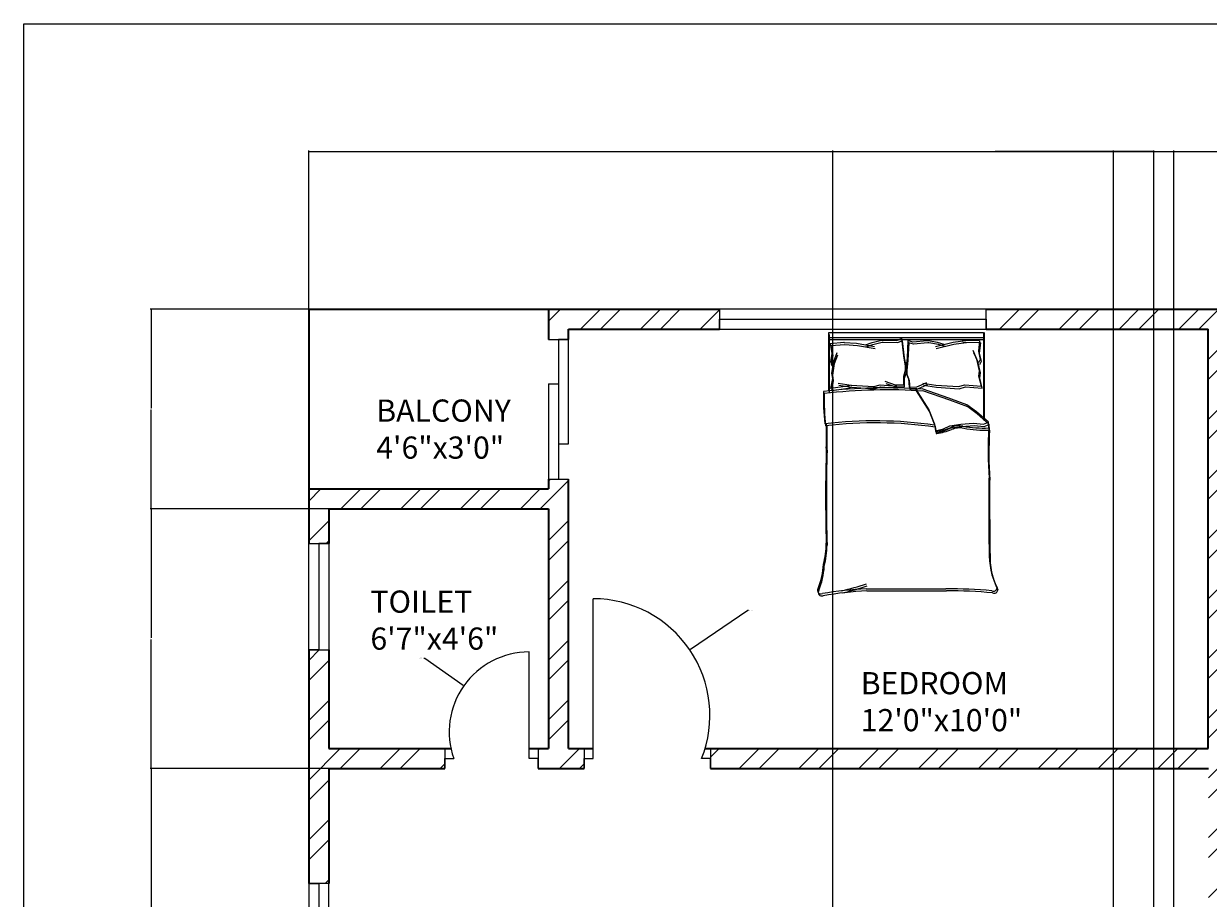
# Model space of a CAD drawing. Units: inches. Extents: x 2064 to 2782, y 1196 to 2299.
# Tile 6 of 11: x 2064 to 2331, y 2102 to 2299. Entities that reach past the tile are written whole.
import ezdxf

# ---------------------------------------------------------------- set-up
doc = ezdxf.new("R2010")
doc.units = ezdxf.units.IN
for name, color, linetype, lineweight in [('A-ANNO-DIMS', 2, 'Continuous', 18), ('A-ANNO-TTLB', 7, 'Continuous', 25), ('A-AREA-IDEN', 7, 'Continuous', 18), ('A-DOOR', 11, 'Continuous', 18), ('A-FURN', 8, 'Continuous', 13), ('A-GLAZ', 151, 'Continuous', 18), ('A-WALL', 7, 'Continuous', 35), ('A-WALL-PATT', 9, 'Continuous', 13)]:
    doc.layers.add(name, color=color, linetype=linetype, lineweight=lineweight)
doc.styles.get("Standard").update_dxf_attribs({"font": 'arial.ttf'})
doc.dimstyles.get("Standard").update_dxf_attribs({"dimtxt": 0.18, "dimasz": 0.18, "dimexe": 0.18, "dimexo": 0.0625, "dimgap": 0.09, "dimtad": 0, "dimtih": 1, "dimtoh": 1, "dimdec": 4, "dimzin": 0, "dimdsep": 46, "dimtxsty": 'Standard', "dimcen": 0.09, "dimadec": 0, "dimazin": 0, "dimtfac": 1, "dimtdec": 4, "dimtofl": 0, "dimtmove": 0, "dimatfit": 3, "dimfxl": 1, "dimtolj": 1, "dimtzin": 0, "dimarcsym": 0})

# ---------------------------------------------------------------- blocks, each defined once
blk = doc.blocks.new('BED-DOUBLE')
for p, q in [((2.53, 46.14), (2.53, 59.33)), ((2.53, 46.14), (2.53, 59.33)), ((2.53, 59.33), (37.35, 59.33)), ((2.7, 45.67), (2.7, 58.87)), ((2.7, 45.67), (2.7, 58.87)), ((37.35, 59.33), (37.35, 39.95)), ((37.35, 59.33), (37.35, 39.95)), ((37.52, 59.33), (37.52, 58.87)), ((37.52, 58.87), (37.52, 39.48)), ((37.52, 58.87), (37.52, 39.48)), ((2.53, 58.22), (37.35, 58.22)), ((2.53, 58.22), (37.35, 58.22)), ((2.7, 57.75), (37.52, 57.75)), ((2.7, 57.75), (37.52, 57.75)), ((2.84, 56.9), (5.96, 57.14)), ((2.84, 56.9), (5.96, 57.14)), ((2.84, 56.92), (3.26, 54.6)), ((2.84, 56.92), (3.26, 54.6)), ((3, 56.45), (3.43, 54.14)), ((3, 56.45), (3.43, 54.14)), ((3.01, 56.44), (6.13, 56.68)), ((3.01, 56.44), (6.13, 56.68)), ((5.96, 57.14), (6.04, 57.13)), ((5.96, 57.14), (6.04, 57.13)), ((6.04, 57.13), (8.82, 56.92)), ((6.04, 57.13), (8.82, 56.92)), ((6.13, 56.68), (6.2, 56.66)), ((6.13, 56.68), (6.2, 56.66)), ((6.2, 56.66), (8.99, 56.45)), ((6.2, 56.66), (8.99, 56.45)), ((8.82, 56.92), (12.82, 56.18)), ((8.82, 56.92), (12.82, 56.18)), ((8.99, 56.45), (12.99, 55.72)), ((8.99, 56.45), (12.99, 55.72)), ((10.82, 56.6), (12.3, 57.13)), ((10.82, 56.6), (12.3, 57.13)), ((10.99, 56.14), (12.46, 56.66)), ((10.99, 56.14), (12.46, 56.66)), ((12.3, 57.13), (14.4, 57.66)), ((12.3, 57.13), (14.4, 57.66)), ((12.46, 56.66), (14.57, 57.19)), ((12.46, 56.66), (14.57, 57.19)), ((14.4, 57.66), (14.64, 57.66)), ((14.4, 57.66), (14.64, 57.66)), ((14.57, 57.19), (14.8, 57.19)), ((14.57, 57.19), (14.8, 57.19)), ((14.64, 57.66), (17.88, 57.55)), ((14.64, 57.66), (17.88, 57.55)), ((14.8, 57.19), (18.04, 57.09)), ((14.8, 57.19), (18.04, 57.09)), ((17.88, 57.55), (18.93, 57.97)), ((17.88, 57.55), (18.93, 57.97)), ((18.04, 57.09), (19.1, 57.51)), ((18.04, 57.09), (19.1, 57.51)), ((18.93, 57.97), (19.35, 54.07)), ((18.93, 57.97), (19.35, 54.07)), ((19.1, 57.51), (19.52, 53.61)), ((19.1, 57.51), (19.52, 53.61)), ((20.38, 57.52), (20.2, 53.6)), ((20.38, 57.52), (20.21, 53.6)), ((20.55, 57.05), (20.37, 53.14)), ((20.55, 57.05), (20.37, 53.14)), ((21.46, 57.16), (20.38, 57.52)), ((21.46, 57.16), (20.38, 57.52)), ((21.63, 56.7), (20.55, 57.05)), ((21.63, 56.7), (20.55, 57.05)), ((24.69, 57.47), (21.46, 57.16)), ((24.69, 57.47), (21.46, 57.16)), ((24.85, 57.01), (21.63, 56.7)), ((24.85, 57.01), (21.63, 56.7)), ((24.92, 57.49), (24.69, 57.47)), ((24.92, 57.49), (24.69, 57.47)), ((25.09, 57.02), (24.85, 57.01)), ((25.09, 57.02), (24.85, 57.01)), ((27.05, 57.09), (24.92, 57.49)), ((27.05, 57.09), (24.92, 57.49)), ((27.22, 56.63), (25.09, 57.02)), ((27.22, 56.63), (25.09, 57.02)), ((30.54, 57.1), (26.59, 56.11)), ((30.54, 57.1), (26.59, 56.11)), ((30.7, 56.63), (26.75, 55.65)), ((30.7, 56.63), (26.75, 55.65)), ((28.56, 56.66), (27.05, 57.09)), ((28.56, 56.66), (27.05, 57.09)), ((28.73, 56.19), (27.22, 56.63)), ((28.73, 56.19), (27.22, 56.63)), ((33.3, 57.48), (30.54, 57.1)), ((33.3, 57.48), (30.54, 57.1)), ((33.47, 57.02), (30.7, 56.63)), ((33.47, 57.02), (30.7, 56.63)), ((36.51, 57.47), (32.57, 57.54)), ((32.57, 57.54), (33.3, 57.48)), ((36.51, 57.47), (32.57, 57.54)), ((32.57, 57.54), (33.3, 57.48)), ((36.68, 57.01), (32.74, 57.08)), ((32.74, 57.08), (33.47, 57.02)), ((36.67, 57.01), (32.74, 57.08)), ((32.74, 57.08), (33.47, 57.02)), ((36.51, 57.47), (36.23, 55.13)), ((36.51, 57.47), (36.23, 55.13)), ((36.68, 57.01), (36.4, 54.67)), ((36.67, 57.01), (36.4, 54.67)), ((3.26, 54.6), (2.94, 52.71)), ((3.26, 54.6), (2.94, 52.71)), ((3.43, 54.14), (3.11, 52.24)), ((3.43, 54.14), (3.11, 52.24)), ((3.68, 52.81), (4.42, 54.81)), ((3.68, 52.81), (4.42, 54.81)), ((3.85, 52.34), (4.58, 54.35)), ((3.85, 52.34), (4.58, 54.35)), ((19.35, 54.07), (19.77, 51.76)), ((19.35, 54.07), (19.77, 51.76)), ((19.52, 53.61), (19.94, 51.29)), ((19.52, 53.61), (19.94, 51.29)), ((20.21, 53.6), (19.93, 51.26)), ((20.2, 53.6), (19.93, 51.26)), ((35.92, 53.32), (35.06, 55.27)), ((35.92, 53.32), (35.06, 55.27)), ((36.09, 52.85), (35.23, 54.8)), ((36.09, 52.85), (35.23, 54.8)), ((36.23, 55.13), (36.67, 53.26)), ((36.23, 55.13), (36.67, 53.26)), ((36.4, 54.67), (36.83, 52.79)), ((36.4, 54.67), (36.83, 52.79)), ((2.94, 52.71), (3.36, 51.97)), ((2.94, 52.71), (3.36, 51.97)), ((3.11, 52.24), (3.53, 51.5)), ((3.11, 52.24), (3.53, 51.5)), ((3.26, 50.18), (3.68, 52.81)), ((3.26, 50.18), (3.68, 52.81)), ((3.43, 49.71), (3.85, 52.34)), ((3.43, 49.71), (3.85, 52.34)), ((19.77, 50.81), (19.35, 49.44)), ((19.77, 50.81), (19.35, 49.44)), ((19.77, 51.76), (19.77, 50.81)), ((19.77, 51.76), (19.77, 50.81)), ((19.93, 51.26), (19.99, 50.32)), ((19.93, 51.26), (19.99, 50.32)), ((19.94, 51.29), (19.94, 50.34)), ((19.94, 51.29), (19.94, 50.34)), ((20.37, 53.14), (20.1, 50.8)), ((20.37, 53.14), (20.1, 50.8)), ((20.1, 50.8), (20.15, 49.85)), ((20.1, 50.8), (20.15, 49.85)), ((36.51, 50.72), (35.92, 53.32)), ((36.51, 50.72), (35.92, 53.32)), ((36.68, 50.25), (36.09, 52.85)), ((36.67, 50.25), (36.09, 52.85)), ((36.67, 53.26), (36.29, 52.5)), ((36.67, 53.26), (36.29, 52.5)), ((36.37, 49.55), (36.51, 50.72)), ((36.37, 49.55), (36.51, 50.72)), ((36.83, 52.79), (36.46, 52.03)), ((36.83, 52.79), (36.46, 52.03)), ((3.05, 46.7), (3.47, 49.02)), ((3.05, 46.7), (3.47, 49.02)), ((3.21, 46.24), (3.64, 48.55)), ((3.21, 46.24), (3.64, 48.55)), ((3.47, 49.02), (3.26, 50.18)), ((3.47, 49.02), (3.26, 50.18)), ((3.64, 48.55), (3.43, 49.71)), ((3.64, 48.55), (3.43, 49.71)), ((17.56, 47.49), (15.27, 48.28)), ((17.56, 47.49), (15.27, 48.28)), ((19.35, 49.44), (19.35, 47.49)), ((19.35, 49.44), (19.35, 47.49)), ((19.94, 50.34), (19.52, 48.97)), ((19.94, 50.34), (19.52, 48.97)), ((19.52, 48.97), (19.52, 47.02)), ((19.52, 48.97), (19.52, 47.02)), ((19.99, 50.32), (20.49, 48.98)), ((19.99, 50.32), (20.49, 48.98)), ((20.15, 49.85), (20.66, 48.51)), ((20.15, 49.85), (20.66, 48.51)), ((20.49, 48.98), (20.62, 47.03)), ((20.49, 48.98), (20.62, 47.03)), ((20.66, 48.51), (20.78, 46.56)), ((20.66, 48.51), (20.78, 46.56)), ((22.4, 47.14), (24.64, 48.08)), ((22.4, 47.14), (24.64, 48.08)), ((36.94, 47.26), (36.37, 49.55)), ((36.94, 47.26), (36.37, 49.55)), ((36.54, 49.08), (36.68, 50.25)), ((36.54, 49.08), (36.67, 50.25)), ((37.1, 46.79), (36.54, 49.08)), ((37.1, 46.79), (36.54, 49.08)), ((6.76, 47.23), (3.05, 46.7)), ((6.76, 47.23), (3.05, 46.7)), ((6.93, 46.76), (3.21, 46.24)), ((6.93, 46.76), (3.21, 46.24)), ((4.65, 47.95), (7.59, 47.46)), ((4.65, 47.95), (7.59, 47.46)), ((4.82, 47.48), (7.75, 47)), ((4.82, 47.48), (7.75, 47)), ((7.59, 47.46), (6.76, 47.23)), ((7.59, 47.46), (6.76, 47.23)), ((7.75, 47), (6.93, 46.76)), ((7.75, 47), (6.93, 46.76)), ((7.59, 47.46), (12.69, 47.15)), ((7.59, 47.46), (12.69, 47.15)), ((7.75, 47), (12.86, 46.68)), ((7.75, 47), (12.86, 46.68)), ((12.69, 47.15), (14.12, 47.55)), ((12.69, 47.15), (14.12, 47.55)), ((12.86, 46.68), (14.29, 47.09)), ((12.86, 46.68), (14.29, 47.09)), ((14.12, 47.55), (17.86, 47.26)), ((14.12, 47.55), (17.86, 47.26)), ((14.29, 47.09), (18.03, 46.79)), ((14.29, 47.09), (18.03, 46.79)), ((17.73, 47.02), (15.44, 47.82)), ((17.73, 47.02), (15.44, 47.82)), ((19.35, 47.49), (17.56, 47.49)), ((19.35, 47.49), (17.56, 47.49)), ((19.52, 47.02), (17.73, 47.02)), ((19.52, 47.02), (17.73, 47.02)), ((20.62, 47.03), (22.4, 47.14)), ((20.62, 47.03), (22.4, 47.14)), ((20.78, 46.56), (22.57, 46.67)), ((20.78, 46.56), (22.57, 46.67)), ((22.05, 46.67), (25.1, 41.94)), ((22.05, 46.67), (25.1, 41.94)), ((22.21, 46.2), (25.26, 41.47)), ((22.21, 46.2), (25.26, 41.47)), ((22.57, 46.67), (24.81, 47.61)), ((22.57, 46.67), (24.81, 47.61)), ((29.61, 44.53), (23.54, 46.67)), ((29.61, 44.53), (23.54, 46.67)), ((29.78, 44.07), (23.7, 46.2)), ((29.78, 44.07), (23.7, 46.2)), ((23.72, 47.95), (26.66, 47.46)), ((23.72, 47.95), (26.66, 47.46)), ((23.89, 47.48), (26.83, 47)), ((23.89, 47.48), (26.83, 47)), ((26.66, 47.46), (31.77, 47.15)), ((26.66, 47.46), (31.77, 47.15)), ((26.83, 47), (31.94, 46.68)), ((26.83, 47), (31.94, 46.68)), ((31.77, 47.15), (33.2, 47.55)), ((31.77, 47.15), (33.2, 47.55)), ((31.94, 46.68), (33.36, 47.09)), ((31.94, 46.68), (33.36, 47.09)), ((33.2, 47.55), (36.94, 47.26)), ((33.2, 47.55), (36.94, 47.26)), ((33.36, 47.09), (37.1, 46.79)), ((33.36, 47.09), (37.1, 46.79)), ((33.67, 43.07), (29.61, 44.53)), ((33.67, 43.07), (29.61, 44.53)), ((33.84, 42.6), (29.78, 44.07)), ((33.84, 42.6), (29.78, 44.07)), ((35.82, 41.49), (33.67, 43.07)), ((35.82, 41.49), (33.67, 43.07)), ((25.1, 41.94), (26.34, 38.67)), ((25.1, 41.94), (26.34, 38.67)), ((25.26, 41.47), (26.51, 38.2)), ((25.26, 41.47), (26.51, 38.2)), ((35.98, 41.02), (33.84, 42.6)), ((35.98, 41.02), (33.84, 42.6)), ((38.52, 39.12), (35.82, 41.49)), ((38.52, 39.12), (35.82, 41.49)), ((38.68, 38.65), (35.98, 41.02)), ((38.68, 38.65), (35.98, 41.02)), ((26.34, 38.67), (26.56, 37.2)), ((26.34, 38.67), (26.56, 37.2)), ((26.51, 38.2), (26.73, 36.74)), ((26.51, 38.2), (26.73, 36.74)), ((26.56, 37.2), (28.37, 37.65)), ((26.56, 37.2), (28.37, 37.65)), ((28.37, 37.65), (29.84, 38.33)), ((28.37, 37.65), (29.84, 38.33)), ((28.54, 37.19), (30, 37.87)), ((28.54, 37.19), (30, 37.87)), ((29.84, 38.33), (32.32, 38.67)), ((29.84, 38.33), (32.32, 38.67)), ((30, 37.87), (32.49, 38.2)), ((30, 37.87), (32.49, 38.2)), ((32.32, 38.67), (35.14, 38.9)), ((32.32, 38.67), (35.14, 38.9)), ((32.49, 38.2), (35.31, 38.43)), ((32.49, 38.2), (35.31, 38.43)), ((35.14, 38.9), (37.4, 38.67)), ((35.14, 38.9), (37.4, 38.67)), ((35.31, 38.43), (37.56, 38.2)), ((35.31, 38.43), (37.56, 38.2)), ((37.4, 38.67), (38.52, 39.12)), ((37.4, 38.67), (38.52, 39.12)), ((37.56, 38.2), (38.68, 38.65)), ((37.56, 38.2), (38.68, 38.65)), ((38.57, 37.85), (38.52, 39.12, 2.82)), ((38.57, 37.85), (38.52, 39.12, 2.82)), ((38.74, 37.38), (38.68, 38.65, 2.82)), ((38.74, 37.38), (38.68, 38.65, 2.82)), ((26.73, 36.74), (28.54, 37.19)), ((26.73, 36.74), (28.54, 37.19)), ((10.97, 1.6), (28.91, 1.6)), ((10.97, 1.6), (28.91, 1.6)), ((11.14, 1.14), (29.07, 1.14)), ((11.14, 1.14), (29.07, 1.14))]:
    blk.add_line(p, q)
for centre, radius, start, end in [((62.04, 44.69), 60.69, 178.7218, 185.604), ((62.04, 44.69), 60.69, 178.7218, 185.604), ((15.56, -73.3), 120.19, 86.0865, 96.7821), ((15.56, -73.3), 120.19, 86.0865, 96.7821), ((62.21, 44.23), 60.69, 178.7218, 185.604), ((62.21, 44.23), 60.69, 178.7218, 185.604), ((15.73, -73.76), 120.19, 86.0865, 96.7821), ((15.73, -73.76), 120.19, 86.0865, 96.7821), ((12.94, -54.55), 94, 81.7845, 96.9006), ((12.94, -54.55), 94, 81.7845, 96.9006), ((13.1, -55.01), 94, 81.7845, 96.9006), ((13.1, -55.01), 94, 81.7845, 96.9006), ((-121.89, 36.62), 123.93, 358.4762, 1.0082), ((-121.89, 36.62), 123.93, 358.4762, 1.0082), ((-121.72, 36.16), 123.93, 358.4762, 1.0082), ((-121.72, 36.16), 123.93, 358.4762, 1.0082), ((22.7, 58.25), 21.6, 280.6617, 289.8806), ((22.7, 58.25), 21.6, 280.6617, 289.8806), ((22.86, 57.79), 21.6, 280.6617, 289.8806), ((22.86, 57.79), 21.6, 280.6617, 289.8806), ((31.87, 33.79), 4.53, 78.6608, 113.7384), ((31.87, 33.79), 4.53, 78.6608, 113.7384), ((32.04, 33.32), 4.53, 78.6608, 113.7384), ((32.04, 33.32), 4.53, 78.6608, 113.7384), ((37.39, 64.18), 26.36, 259.8763, 272.5657), ((37.39, 64.18), 26.36, 259.8763, 272.5657), ((37.56, 63.72), 26.36, 259.8763, 272.5657), ((37.56, 63.72), 26.36, 259.8763, 272.5657), ((132.79, 32.88), 94.35, 176.9791, 183.8365), ((132.79, 32.88), 94.35, 176.9791, 183.8365), ((132.95, 32.41), 94.35, 176.9791, 183.8365), ((132.95, 32.41), 94.35, 176.9791, 183.8365), ((26.69, 37.16), 0.134, 160.2464, 271.1377), ((26.69, 37.16), 0.134, 160.2464, 271.1377), ((26.86, 36.69), 0.134, 160.2464, 271.1377), ((26.86, 36.69), 0.134, 160.2464, 271.1377), ((353.21, 22.46), 351.38, 178.2277, 181.7185), ((353.21, 22.46), 351.38, 178.2277, 181.7185), ((353.38, 21.99), 351.38, 178.2277, 181.7185), ((353.38, 21.99), 351.38, 178.2277, 181.7185), ((-3284.8, 9.92), 3323.5, 0.00217, 0.28689), ((-3284.8, 9.92), 3323.5, 0.00217, 0.28689), ((-3284.64, 9.46), 3323.5, 0.00217, 0.28689), ((-3284.64, 9.46), 3323.5, 0.00217, 0.28689), ((-19.6, 12.33), 21.59, 346.0648, 358.9113), ((-19.6, 12.33), 21.59, 346.0648, 358.9113), ((-19.43, 11.87), 21.59, 346.0648, 358.9113), ((-19.43, 11.87), 21.59, 346.0648, 358.9113), ((55.48, 9.31), 16.8, 177.4714, 206.4681), ((55.48, 9.31), 16.8, 177.4714, 206.4681), ((55.65, 8.84), 16.8, 177.4714, 206.4681), ((55.65, 8.84), 16.8, 177.4714, 206.4681), ((-15.78, 8.14), 17.17, 337.9751, 356.652), ((-15.78, 8.14), 17.17, 337.9751, 356.652), ((-15.61, 7.67), 17.17, 337.9751, 356.652), ((-15.61, 7.67), 17.17, 337.9751, 356.652), ((-12.55, 76.61), 77.56, 283.3832, 287.7053), ((-12.55, 76.61), 77.56, 283.3832, 287.7053), ((0.79, 1.26), 0.793, 146.1736, 293.4781), ((0.79, 1.26), 0.793, 146.1736, 293.4781), ((0.96, 0.79), 0.793, 146.1736, 293.4781), ((0.96, 0.79), 0.793, 146.1736, 293.4781), ((15.61, -86.98), 88.71, 92.9958, 99.4091), ((15.61, -86.98), 88.71, 92.9958, 99.4091), ((15.78, -87.45), 88.71, 92.9958, 99.4091), ((15.78, -87.45), 88.71, 92.9958, 99.4091), ((-12.38, 76.14), 77.56, 283.3832, 287.7053), ((-12.38, 76.14), 77.56, 283.3832, 287.7053), ((29.98, -95.32), 96.92, 84.4998, 90.6351), ((29.98, -95.32), 96.92, 84.4998, 90.6351), ((30.15, -95.78), 96.92, 84.4998, 90.6351), ((30.15, -95.78), 96.92, 84.4998, 90.6351), ((39.64, 1.87), 0.803, 242.6588, 356.02), ((39.64, 1.87), 0.803, 242.6588, 356.02), ((39.81, 1.41), 0.803, 242.6588, 356.02), ((39.81, 1.41), 0.803, 242.6588, 356.02)]:
    blk.add_arc(centre, radius, start, end)
blk = doc.blocks.new('WIN-60IN')
for p, q in [((0, 4.5), (0, 0)), ((60, 4.5), (0, 4.5)), ((60, 2.25), (60, 4.5)), ((60, 4.5), (60, 0)), ((0, 0), (0, 2.25)), ((0, 2.25), (60, 2.25)), ((0, 0), (60, 0))]:
    blk.add_line(p, q)
blk = doc.blocks.new('*D22')
at = {"layer": 'A-ANNO-DIMS', "color": 0, "lineweight": -2, "transparency": 16777216}
for p, q in [((2128.17, 2234.35), (2128.17, 2269.97)), ((2128.35, 2269.79), (2390.38, 2269.79)), ((2652.99, 2269.79), (2390.96, 2269.79)), ((2653.17, 2234.35), (2653.17, 2269.97))]:
    blk.add_line(p, q, dxfattribs=at)
at = {"layer": 'A-ANNO-DIMS', "color": 0, "transparency": 16777216}
for points in [[(2128.35, 2269.82), (2128.35, 2269.76), (2128.17, 2269.79)], [(2652.99, 2269.82), (2652.99, 2269.76), (2653.17, 2269.79)]]:
    blk.add_solid(points, dxfattribs=at)
at = {"layer": 'Defpoints', "color": 0, "transparency": 16777216}
for p in [(2653.17, 2269.79), (2128.17, 2234.29), (2653.17, 2234.29)]:
    blk.add_point(p, dxfattribs=at)
at = {"layer": 'A-ANNO-DIMS', "color": 0, "transparency": 16777216, "insert": (2390.67, 2269.79), "char_height": 0.18, "attachment_point": 5}
blk.add_mtext('\\A1;525', dxfattribs=at)
blk = doc.blocks.new('*D26')
at = {"layer": 'A-ANNO-DIMS', "color": 0, "lineweight": -2, "transparency": 16777216}
for p, q in [((2246.18, 1643.35), (2246.18, 2269.97)), ((2246.36, 2269.79), (2281.92, 2269.79)), ((2318.27, 2269.79), (2282.71, 2269.79)), ((2318.45, 1640.85), (2318.45, 2269.97))]:
    blk.add_line(p, q, dxfattribs=at)
at = {"layer": 'A-ANNO-DIMS', "color": 0, "transparency": 16777216}
for points in [[(2246.36, 2269.82), (2246.36, 2269.76), (2246.18, 2269.79)], [(2318.27, 2269.82), (2318.27, 2269.76), (2318.45, 2269.79)]]:
    blk.add_solid(points, dxfattribs=at)
at = {"layer": 'Defpoints', "color": 0, "transparency": 16777216}
for p in [(2318.45, 2269.79), (2246.18, 1643.29), (2318.45, 1640.79)]:
    blk.add_point(p, dxfattribs=at)
at = {"layer": 'A-ANNO-DIMS', "color": 0, "transparency": 16777216, "insert": (2282.32, 2269.79), "char_height": 0.18, "attachment_point": 5}
blk.add_mtext('\\A1;72.27', dxfattribs=at)
blk = doc.blocks.new('*D32')
at = {"layer": 'A-ANNO-DIMS', "color": 0, "lineweight": -2, "transparency": 16777216}
for p, q in [((2132.61, 2130.79), (2092.49, 2130.79)), ((2092.67, 2130.61), (2092.67, 2067.97)), ((2092.67, 2004.97), (2092.67, 2067.61)), ((2132.61, 2004.79), (2092.49, 2004.79))]:
    blk.add_line(p, q, dxfattribs=at)
at = {"layer": 'A-ANNO-DIMS', "color": 0, "transparency": 16777216}
for points in [[(2092.64, 2130.61), (2092.7, 2130.61), (2092.67, 2130.79)], [(2092.64, 2004.97), (2092.7, 2004.97), (2092.67, 2004.79)]]:
    blk.add_solid(points, dxfattribs=at)
at = {"layer": 'Defpoints', "color": 0, "transparency": 16777216}
for p in [(2092.67, 2130.79), (2132.67, 2130.79), (2132.67, 2004.79)]:
    blk.add_point(p, dxfattribs=at)
at = {"layer": 'A-ANNO-DIMS', "color": 0, "transparency": 16777216, "insert": (2092.67, 2067.79), "char_height": 0.18, "attachment_point": 5}
blk.add_mtext('\\A1;126', dxfattribs=at)
blk = doc.blocks.new('*D33')
at = {"layer": 'A-ANNO-DIMS', "color": 0, "lineweight": -2, "transparency": 16777216}
for p, q in [((2132.61, 2189.29), (2092.49, 2189.29)), ((2092.67, 2189.11), (2092.67, 2160.22)), ((2092.67, 2130.97), (2092.67, 2159.86)), ((2132.61, 2130.79), (2092.49, 2130.79))]:
    blk.add_line(p, q, dxfattribs=at)
at = {"layer": 'A-ANNO-DIMS', "color": 0, "transparency": 16777216}
for points in [[(2092.64, 2189.11), (2092.7, 2189.11), (2092.67, 2189.29)], [(2092.64, 2130.97), (2092.7, 2130.97), (2092.67, 2130.79)]]:
    blk.add_solid(points, dxfattribs=at)
at = {"layer": 'Defpoints', "color": 0, "transparency": 16777216}
for p in [(2092.67, 2189.29), (2132.67, 2189.29), (2132.67, 2130.79)]:
    blk.add_point(p, dxfattribs=at)
at = {"layer": 'A-ANNO-DIMS', "color": 0, "transparency": 16777216, "insert": (2092.67, 2160.04), "char_height": 0.18, "attachment_point": 5}
blk.add_mtext('\\A1;58.5', dxfattribs=at)
blk = doc.blocks.new('*D34')
at = {"layer": 'A-ANNO-DIMS', "color": 0, "lineweight": -2, "transparency": 16777216}
for p, q in [((2128.11, 2234.29), (2092.49, 2234.29)), ((2092.67, 2234.11), (2092.67, 2211.97)), ((2092.67, 2189.47), (2092.67, 2211.61)), ((2132.61, 2189.29), (2092.49, 2189.29))]:
    blk.add_line(p, q, dxfattribs=at)
at = {"layer": 'A-ANNO-DIMS', "color": 0, "transparency": 16777216}
for points in [[(2092.64, 2234.11), (2092.7, 2234.11), (2092.67, 2234.29)], [(2092.64, 2189.47), (2092.7, 2189.47), (2092.67, 2189.29)]]:
    blk.add_solid(points, dxfattribs=at)
at = {"layer": 'Defpoints', "color": 0, "transparency": 16777216}
for p in [(2092.67, 2234.29), (2128.17, 2234.29), (2132.67, 2189.29)]:
    blk.add_point(p, dxfattribs=at)
at = {"layer": 'A-ANNO-DIMS', "color": 0, "transparency": 16777216, "insert": (2092.67, 2211.79), "char_height": 0.18, "attachment_point": 5}
blk.add_mtext('\\A1;45', dxfattribs=at)
blk = doc.blocks.new('*D35')
at = {"layer": 'A-ANNO-DIMS', "color": 0, "lineweight": -2, "transparency": 16777216}
for p, q in [((2309.4, 1932.85), (2309.4, 2269.97)), ((2309.58, 2269.79), (2347.37, 2269.79)), ((2385.94, 2269.79), (2348.16, 2269.79)), ((2386.12, 1856.35), (2386.12, 2269.97))]:
    blk.add_line(p, q, dxfattribs=at)
at = {"layer": 'A-ANNO-DIMS', "color": 0, "transparency": 16777216}
for points in [[(2309.58, 2269.82), (2309.58, 2269.76), (2309.4, 2269.79)], [(2385.94, 2269.82), (2385.94, 2269.76), (2386.12, 2269.79)]]:
    blk.add_solid(points, dxfattribs=at)
at = {"layer": 'Defpoints', "color": 0, "transparency": 16777216}
for p in [(2386.12, 2269.79), (2309.4, 1932.79), (2386.12, 1856.29)]:
    blk.add_point(p, dxfattribs=at)
at = {"layer": 'A-ANNO-DIMS', "color": 0, "transparency": 16777216, "insert": (2347.76, 2269.79), "char_height": 0.18, "attachment_point": 5}
blk.add_mtext('\\A1;76.72', dxfattribs=at)
blk = doc.blocks.new('*D39')
at = {"layer": 'A-ANNO-DIMS', "color": 0, "lineweight": -2, "transparency": 16777216}
for p, q in [((2322.95, 1645.35), (2322.95, 2269.97)), ((2323.13, 2269.79), (2333.59, 2269.79)), ((2344.97, 2269.79), (2334.51, 2269.79)), ((2345.15, 1645.35), (2345.15, 2269.97))]:
    blk.add_line(p, q, dxfattribs=at)
at = {"layer": 'A-ANNO-DIMS', "color": 0, "transparency": 16777216}
for points in [[(2323.13, 2269.82), (2323.13, 2269.76), (2322.95, 2269.79)], [(2344.97, 2269.82), (2344.97, 2269.76), (2345.15, 2269.79)]]:
    blk.add_solid(points, dxfattribs=at)
at = {"layer": 'Defpoints', "color": 0, "transparency": 16777216}
for p in [(2345.15, 2269.79), (2322.95, 1645.29), (2345.15, 1645.29)]:
    blk.add_point(p, dxfattribs=at)
at = {"layer": 'A-ANNO-DIMS', "color": 0, "transparency": 16777216, "insert": (2334.05, 2269.79), "char_height": 0.18, "attachment_point": 5}
blk.add_mtext('\\A1;22.194', dxfattribs=at)
blk = doc.blocks.new('*D48')
at = {"layer": 'A-ANNO-DIMS', "color": 0, "lineweight": -2, "transparency": 16777216}
for p, q in [((2227.01, 2166.36), (2214.11, 2157.61)), ((2227.19, 2166.36), (2227.01, 2166.36)), ((2192.12, 2142.76), (2192.3, 2142.76)), ((2192.21, 2142.67), (2192.21, 2142.85))]:
    blk.add_line(p, q, dxfattribs=at)
at = {"layer": 'A-ANNO-DIMS', "color": 0, "transparency": 16777216}
blk.add_solid([(2214.1, 2157.64), (2214.13, 2157.59), (2213.96, 2157.51)], dxfattribs=at)
at = {"layer": 'Defpoints', "color": 0, "transparency": 16777216}
for p in [(2213.96, 2157.51), (2192.21, 2142.76)]:
    blk.add_point(p, dxfattribs=at)
at = {"layer": 'A-ANNO-DIMS', "color": 0, "transparency": 16777216, "insert": (2227.67, 2166.36), "char_height": 0.18, "attachment_point": 5}
blk.add_mtext('\\A1;R26.28', dxfattribs=at)
blk = doc.blocks.new('*D50')
at = {"layer": 'A-ANNO-DIMS', "color": 0, "lineweight": -2, "transparency": 16777216}
for p, q in [((2154.1, 2155.68), (2154.28, 2155.68)), ((2154.28, 2155.68), (2162.95, 2149.54)), ((2177.8, 2138.94), (2177.8, 2139.12)), ((2177.71, 2139.03), (2177.89, 2139.03))]:
    blk.add_line(p, q, dxfattribs=at)
at = {"layer": 'A-ANNO-DIMS', "color": 0, "transparency": 16777216}
blk.add_solid([(2162.97, 2149.56), (2162.94, 2149.52), (2163.1, 2149.44)], dxfattribs=at)
at = {"layer": 'Defpoints', "color": 0, "transparency": 16777216}
for p in [(2163.1, 2149.44), (2177.8, 2139.03)]:
    blk.add_point(p, dxfattribs=at)
at = {"layer": 'A-ANNO-DIMS', "color": 0, "transparency": 16777216, "insert": (2153.55, 2155.68), "char_height": 0.18, "attachment_point": 5}
blk.add_mtext('\\A1;R18.013', dxfattribs=at)

msp = doc.modelspace()

# ---------------------------------------------------------------- hatches: boundary and pattern name
at = {"layer": 'A-WALL-PATT'}
h = msp.add_hatch(dxfattribs=at)
h.set_pattern_fill('ANSI32', color=256)
h.paths.add_polyline_path([(2489.7688, 2189.2917), (2574.5454, 2189.2917), (2574.5454, 2191.5417), (2574.5454, 2193.7917), (2570.6691, 2193.7917), (2570.6691, 2197.3052), (2568.4191, 2197.3052), (2566.1691, 2197.3052), (2566.1691, 2193.7917), (2494.1691, 2193.7917), (2494.1691, 2229.7917), (2523.2441, 2229.7917), (2523.2441, 2234.2917), (2471.2886, 2234.2917), (2471.2886, 2229.7917), (2489.6691, 2229.7917), (2489.6691, 2193.7917), (2417.6691, 2193.7917), (2417.6691, 2197.0632), (2415.4191, 2197.0632), (2413.1691, 2197.0632), (2413.1691, 2193.7917), (2406.8865, 2193.7917), (2406.8865, 2189.2917), (2485.2688, 2189.2917), (2485.2688, 2063.2917), (2369.1629, 2063.2917), (2369.1629, 2058.7917), (2386.1222, 2058.7917), (2386.1222, 1856.2917), (2382.1576, 1856.2917), (2382.1576, 1851.7917), (2394.9764, 1851.7917), (2394.9764, 1854.0417), (2394.9764, 1856.2917), (2390.6222, 1856.2917), (2390.6222, 2058.7917), (2485.2688, 2058.7917), (2493.762, 2058.7917), (2493.762, 2061.0417), (2493.762, 2063.2917), (2489.7688, 2063.2917)])
h.paths.add_polyline_path([(2447.2886, 2234.2917), (2413.1691, 2234.2917), (2413.1691, 2217.3799), (2417.6691, 2217.3799), (2417.6691, 2229.7917), (2447.2886, 2229.7917)], flags=17)
h.paths.add_polyline_path([(2570.6691, 2234.2917), (2547.2441, 2234.2917), (2547.2441, 2229.7917), (2566.1691, 2229.7917), (2566.1691, 2216.5615), (2570.6691, 2216.5615)], flags=17)
h.paths.add_polyline_path([(2653.1691, 2189.2917), (2653.1691, 2193.7917), (2640.8843, 2193.7917), (2640.8843, 2189.2917), (2648.6691, 2189.2917), (2648.6691, 2162.7138), (2653.1691, 2162.7138)])
h.paths.add_polyline_path([(2653.1691, 2102.7138), (2648.6691, 2102.7138), (2648.6691, 2063.2917), (2526.7281, 2063.2917), (2526.7281, 2058.7917), (2541.1691, 2058.7917), (2541.1691, 1993.2917), (2545.6691, 1993.2917), (2545.6691, 1997.7917), (2545.6691, 2058.7917), (2648.6691, 2058.7917), (2648.6691, 2050.1099), (2653.1691, 2050.1099)])
h.paths.add_polyline_path([(2600.6691, 1856.2917), (2493.4607, 1856.2917), (2493.4607, 1851.7917), (2596.1691, 1851.7917), (2596.1691, 1695.7917), (2594.0816, 1695.7917), (2594.0816, 1691.2917), (2614.7905, 1691.2917), (2614.7905, 1645.2917), (2536.7905, 1645.2917), (2536.7905, 1691.2917), (2539.332, 1691.2917), (2539.332, 1693.5417), (2539.332, 1695.7917), (2452.1691, 1695.7917), (2452.1691, 1851.7917), (2456.0775, 1851.7917), (2456.0775, 1856.2917), (2427.1536, 1856.2917), (2427.1536, 1851.7917), (2447.6691, 1851.7917), (2447.6691, 1695.7917), (2447.6691, 1645.2917), (2405.1469, 1645.2917), (2405.1469, 1640.7917), (2452.1691, 1640.7917), (2452.1691, 1645.2917), (2452.1691, 1691.2917), (2534.7905, 1691.2917), (2534.7905, 1645.2917), (2534.7905, 1643.2917), (2614.7905, 1643.2917), (2616.7905, 1643.2917), (2616.7905, 1691.2917), (2622.4029, 1691.2917), (2622.4029, 1693.7143), (2622.4029, 1695.7917), (2600.6691, 1695.7917), (2600.6691, 1779.7917), (2648.6691, 1779.7917), (2648.6691, 1695.7917), (2646.4029, 1695.7917), (2646.4029, 1691.2917), (2653.1691, 1691.2917), (2653.1691, 1906.3508), (2648.6691, 1906.3508), (2648.6691, 1856.2917), (2648.6691, 1784.2917), (2600.6691, 1784.2917)])
h.paths.add_polyline_path([(2322.9532, 1819.5181), (2320.7032, 1819.5181), (2318.4532, 1819.5181), (2318.4532, 1695.7917), (2242.7664, 1695.7917), (2242.7664, 1691.2917), (2318.4532, 1691.2917), (2318.4532, 1640.7917), (2322.9532, 1640.7917), (2345.1469, 1640.7917), (2345.1469, 1643.0417), (2345.1469, 1645.2917), (2322.9532, 1645.2917), (2322.9532, 1691.2917), (2322.9532, 1695.7917)])
h.paths.add_polyline_path([(2166.1825, 1691.2917), (2164.1825, 1691.2917), (2164.1825, 1643.2917), (2166.1825, 1643.2917), (2246.1825, 1643.2917), (2246.1825, 1645.2917), (2246.1825, 1691.2917), (2244.1825, 1691.2917), (2244.1825, 1645.2917), (2166.1825, 1645.2917)])
h.paths.add_polyline_path([(2309.404, 1932.7917), (2204.1691, 1932.7917), (2204.1691, 1960.0962), (2199.6691, 1960.0962), (2199.6691, 1932.7917), (2132.6691, 1932.7917), (2132.6691, 1951.0737), (2128.1691, 1951.0737), (2128.1691, 1910.0412), (2132.6691, 1910.0412), (2132.6691, 1928.2917), (2304.904, 1928.2917), (2304.904, 1856.2917), (2304.904, 1851.7917), (2318.4532, 1851.7917), (2318.4532, 1848.8308), (2322.9532, 1848.8308), (2322.9532, 1851.7917), (2347.7631, 1851.7917), (2347.7631, 1856.2917), (2309.404, 1856.2917)])
h.paths.add_polyline_path([(2132.6691, 2044.9092), (2130.4191, 2044.9092), (2128.1691, 2044.9092), (2128.1691, 1987.0737), (2132.6691, 1987.0737), (2132.6691, 2004.7917), (2199.6691, 2004.7917), (2204.1691, 2004.7917), (2204.1691, 2009.2917), (2132.6691, 2009.2917)])
h.paths.add_polyline_path([(2186.6691, 2195.9329), (2184.4191, 2195.9329), (2184.4191, 2195.8929), (2182.1691, 2195.9329), (2182.1691, 2193.7917), (2128.1691, 2193.7917), (2128.1691, 2181.4967), (2132.6691, 2181.4967), (2132.6691, 2182.7769), (2132.6691, 2189.2917), (2182.1691, 2189.2917), (2182.1691, 2135.2917), (2179.804, 2135.2917), (2179.804, 2130.7917), (2190.215, 2130.7917), (2190.215, 2133.0417), (2190.215, 2135.2917), (2186.6691, 2135.2917)])
h.paths.add_polyline_path([(2340.0628, 2189.2917), (2340.0628, 2191.5417), (2340.0628, 2193.7917), (2335.1691, 2193.7917), (2335.1691, 2234.2917), (2280.6746, 2234.2917), (2280.6746, 2229.7917), (2330.6691, 2229.7917), (2330.6691, 2193.7917), (2330.6691, 2135.2917), (2218.6309, 2135.2917), (2218.6309, 2130.7917), (2330.7688, 2130.7917), (2330.7688, 2008.4023), (2335.2688, 2008.4023), (2335.2688, 2058.7917), (2338.9208, 2058.7917), (2338.9208, 2061.0417), (2338.9208, 2063.2917), (2335.2688, 2063.2917), (2335.2688, 2189.2917)])
h.paths.add_polyline_path([(2220.6746, 2234.2917), (2182.1691, 2234.2917), (2182.1691, 2227.4187), (2186.6691, 2227.4187), (2186.6691, 2229.7917), (2220.6746, 2229.7917), (2220.6746, 2232.0417)])
h.paths.add_polyline_path([(2158.8146, 2135.2917), (2132.6691, 2135.2917), (2132.6691, 2157.4967), (2128.1691, 2157.4967), (2128.1691, 2104.9092), (2132.6691, 2104.9092), (2132.6691, 2130.7917), (2158.8146, 2130.7917), (2158.8146, 2133.0417)])
h.paths.add_polyline_path([(2396.0464, 2062.2045), (2434.8868, 2062.2045), (2434.8868, 2080.8619), (2396.0464, 2080.8619)], flags=24)
h.paths.add_polyline_path([(2196.1396, 1653.3449), (2232.023, 1653.3449), (2232.023, 1672.0022), (2196.1396, 1672.0022)], flags=25)

# ---------------------------------------------------------------- linework, layer by layer
at = {"layer": 'A-ANNO-TTLB'}
msp.add_lwpolyline([(2063.9994, 2298.574), (2782.0941, 2298.574), (2782.0941, 1490.6238), (2063.9994, 1490.6238)], close=True, dxfattribs=at)
at = {"layer": 'A-DOOR'}
for p, q in [((2192.215, 2133.0417), (2192.215, 2169.0417)), ((2177.804, 2133.0417), (2177.804, 2157.0417)), ((2158.8146, 2135.2917), (2158.8146, 2130.7917)), ((2179.804, 2135.2917), (2179.804, 2130.7917)), ((2190.215, 2135.2917), (2190.215, 2130.7917)), ((2218.6309, 2135.2917), (2218.6309, 2130.7917)), ((2158.8146, 2130.7917), (2158.8146, 2133.0417)), ((2158.8146, 2133.0417), (2160.8146, 2133.0417)), ((2179.804, 2133.0417), (2177.804, 2133.0417)), ((2179.804, 2130.7917), (2179.804, 2133.0417)), ((2190.215, 2130.7917), (2190.215, 2133.0417)), ((2190.215, 2133.0417), (2192.215, 2133.0417)), ((2218.6309, 2133.0417), (2216.6309, 2133.0417)), ((2218.6309, 2130.7917), (2218.6309, 2133.0417))]:
    msp.add_line(p, q, dxfattribs=at)
for centre, radius, start, end in [((2192.215, 2142.762), 26.2797, 338.291872, 90), ((2177.804, 2139.0284), 18.0133, 90, 199.411304)]:
    msp.add_arc(centre, radius, start, end, dxfattribs=at)
at = {"layer": 'A-GLAZ'}
for p, q in [((2220.6746, 2234.2917), (2220.6746, 2229.7917)), ((2280.6746, 2234.2917), (2220.6746, 2234.2917)), ((2280.6746, 2229.7917), (2280.6746, 2234.2917)), ((2220.6746, 2229.7917), (2220.6746, 2232.0417)), ((2220.6746, 2232.0417), (2280.6746, 2232.0417)), ((2220.6746, 2229.7917), (2280.6746, 2229.7917)), ((2280.6746, 2232.0417), (2280.6746, 2229.7917)), ((2182.1691, 2227.4187), (2186.6691, 2227.4187)), ((2186.6691, 2227.4187), (2184.4191, 2227.4187)), ((2184.4191, 2227.4187), (2184.4191, 2195.8929)), ((2186.6691, 2203.9446), (2186.6691, 2227.4187)), ((2182.1691, 2217.4442), (2182.1691, 2195.9329)), ((2182.1691, 2217.4442), (2184.4191, 2217.4442)), ((2184.4191, 2203.9446), (2186.6691, 2203.9446)), ((2184.4191, 2195.8929), (2182.1691, 2195.9329)), ((2182.1691, 2195.9329), (2186.6691, 2195.9329)), ((2132.6691, 2182.7769), (2132.6691, 2157.4967)), ((2128.1691, 2181.4967), (2132.6691, 2181.4967)), ((2128.1691, 2157.4967), (2128.1691, 2181.4967)), ((2132.6691, 2181.4967), (2130.4191, 2181.4967)), ((2130.4191, 2181.4967), (2130.4191, 2157.4967)), ((2130.4191, 2157.4967), (2128.1691, 2157.4967)), ((2128.1691, 2157.4967), (2132.6691, 2157.4967))]:
    msp.add_line(p, q, dxfattribs=at)
at = {"layer": 'A-WALL'}
for p, q in [((2128.1691, 2234.2917), (2220.6746, 2234.2917)), ((2128.1691, 2234.2917), (2128.1691, 2181.4967)), ((2182.1691, 2234.2917), (2182.1691, 2227.4187)), ((2280.6746, 2234.2917), (2447.2886, 2234.2917)), ((2186.6691, 2229.7917), (2220.6746, 2229.7917)), ((2186.6691, 2227.4187), (2186.6691, 2229.7917)), ((2186.6691, 2227.4187), (2186.6691, 2229.7917)), ((2280.6746, 2229.7917), (2330.6691, 2229.7917)), ((2330.6691, 2193.7917), (2330.6691, 2229.7917)), ((2330.6691, 2135.2917), (2330.6691, 2229.7917)), ((2182.1691, 2195.9329), (2182.1691, 2193.7917)), ((2186.6691, 2135.2917), (2186.6691, 2195.9329)), ((2186.6691, 2193.7917), (2186.6691, 2195.9329)), ((2128.1691, 2193.7917), (2182.1691, 2193.7917)), ((2132.6691, 2189.2917), (2182.1691, 2189.2917)), ((2132.6691, 2189.2917), (2132.6691, 2181.4967)), ((2182.1691, 2189.2917), (2182.1691, 2135.2917)), ((2128.1691, 2157.4967), (2128.1691, 2104.9092)), ((2132.6691, 2157.4967), (2132.6691, 2135.2917)), ((2132.6691, 2135.2917), (2160.1825, 2135.2917)), ((2177.804, 2135.2917), (2182.1691, 2135.2917)), ((2186.6691, 2135.2917), (2192.215, 2135.2917)), ((2217.4106, 2135.2917), (2330.6691, 2135.2917)), ((2132.6691, 2130.7917), (2158.8146, 2130.7917)), ((2132.6691, 2130.7917), (2132.6691, 2104.9092)), ((2179.804, 2130.7917), (2190.215, 2130.7917)), ((2218.6309, 2130.7917), (2330.7688, 2130.7917))]:
    msp.add_line(p, q, dxfattribs=at)

# ---------------------------------------------------------------- block references
at = {"layer": 'A-FURN'}
msp.add_blockref('BED-DOUBLE', (2242.7167, 2169.6588), dxfattribs=at)
at = {"layer": 'A-GLAZ', "rotation": 270}
msp.add_blockref('WIN-60IN', (2128.1691, 2104.9092), dxfattribs=at)

# ---------------------------------------------------------------- texts
at = {"layer": 'A-AREA-IDEN', "char_height": 5, "attachment_point": 1}
for s, width, insert in [('BALCONY\\P4\'6"x3\'0"', 95.384213, (2143.3747, 2213.9131)), ('TOILET\\P6\'7"x4\'6"', 90.19418, (2142.0622, 2170.8876)), ('BEDROOM\\P12\'0"x10\'0"', 151.009925, (2252.4513, 2152.5191))]:
    msp.add_mtext_dynamic_manual_height_columns(s, width=width, gutter_width=12.5, heights=[0], dxfattribs=dict(at, insert=insert))

# ---------------------------------------------------------------- dimensions: what is measured, and where the dimension line sits
at = {"layer": 'A-ANNO-DIMS'}
for base, p1, p2, override, picture, middle in [((2653.1691, 2269.7917), (2128.1691, 2234.2917), (2653.1691, 2234.2917), {"dimdec": 0, "dimlfac": 1, "dimrnd": 0, "dimzin": 0, "dimdsep": 46, "dimlunit": 2}, '*D22', (2390.6691, 2269.7917)), ((2318.4532, 2269.7917), (2246.1825, 1643.2917), (2318.4532, 1640.7917), {"dimdec": 2, "dimlfac": 1, "dimrnd": 0, "dimzin": 0, "dimdsep": 46, "dimlunit": 2}, '*D26', (2282.3178, 2269.7917)), ((2386.1222, 2269.7917), (2309.404, 1932.7917), (2386.1222, 1856.2917), {"dimdec": 2, "dimlfac": 1, "dimrnd": 0, "dimzin": 0, "dimdsep": 46, "dimlunit": 2}, '*D35', (2347.7631, 2269.7917)), ((2345.1469, 2269.7917), (2322.9532, 1645.2917), (2345.1469, 1645.2917), {"dimdec": 3, "dimlfac": 1, "dimrnd": 0, "dimzin": 0, "dimdsep": 46, "dimlunit": 2}, '*D39', (2334.0501, 2269.7917))]:
    dim = msp.add_linear_dim(base=base, p1=p1, p2=p2, dimstyle='Standard', override=override, dxfattribs=at)
    dim.commit()
    dim.dimension.update_dxf_attribs({"geometry": picture, "text_midpoint": middle})
for base, p1, p2, override, picture, middle in [((2092.6691, 2234.2917), (2132.6691, 2189.2917), (2128.1691, 2234.2917), {"dimdec": 0, "dimlfac": 1, "dimrnd": 0, "dimzin": 0, "dimdsep": 46, "dimlunit": 2}, '*D34', (2092.6691, 2211.7917)), ((2092.6691, 2189.2917), (2132.6691, 2130.7917), (2132.6691, 2189.2917), {"dimdec": 1, "dimlfac": 1, "dimrnd": 0, "dimzin": 0, "dimdsep": 46, "dimlunit": 2}, '*D33', (2092.6691, 2160.0417)), ((2092.6691, 2130.7917), (2132.6691, 2004.7917), (2132.6691, 2130.7917), {"dimdec": 0, "dimlfac": 1, "dimrnd": 0, "dimzin": 0, "dimdsep": 46, "dimlunit": 2}, '*D32', (2092.6691, 2067.7917))]:
    dim = msp.add_linear_dim(base=base, p1=p1, p2=p2, angle=90, dimstyle='Standard', override=override, dxfattribs=at)
    dim.commit()
    dim.dimension.update_dxf_attribs({"geometry": picture, "text_midpoint": middle})
for center, mpoint, override, picture, middle in [((2192.215, 2142.762), (2213.9642, 2157.5131), {"dimdec": 2, "dimlfac": 1, "dimrnd": 0, "dimzin": 0, "dimdsep": 46, "dimlunit": 2}, '*D48', (2227.6737, 2166.3638)), ((2177.804, 2139.0284), (2163.1017, 2149.4362), {"dimdec": 3, "dimlfac": 1, "dimrnd": 0, "dimzin": 0, "dimdsep": 46, "dimlunit": 2}, '*D50', (2153.5506, 2155.6809))]:
    dim = msp.add_radius_dim(center=center, mpoint=mpoint, dimstyle='Standard', override=override, dxfattribs=at)
    dim.commit()
    dim.dimension.update_dxf_attribs({"geometry": picture, "text_midpoint": middle, "dimtype": 164})

doc.saveas('drawing.dxf')
